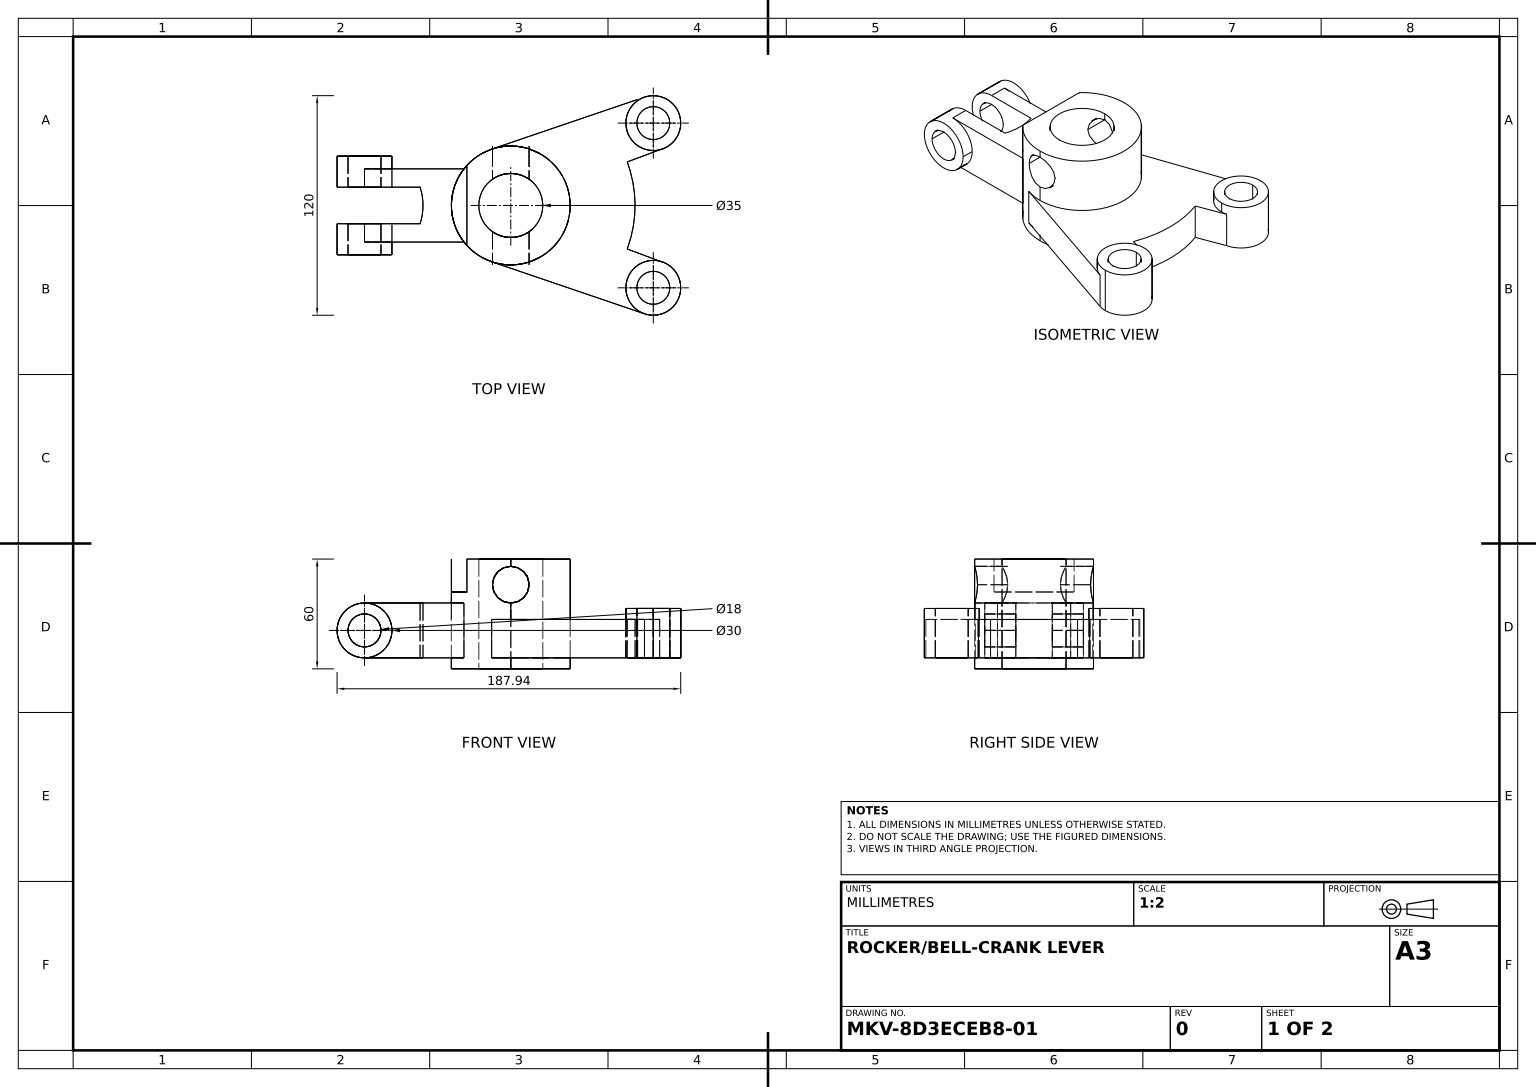
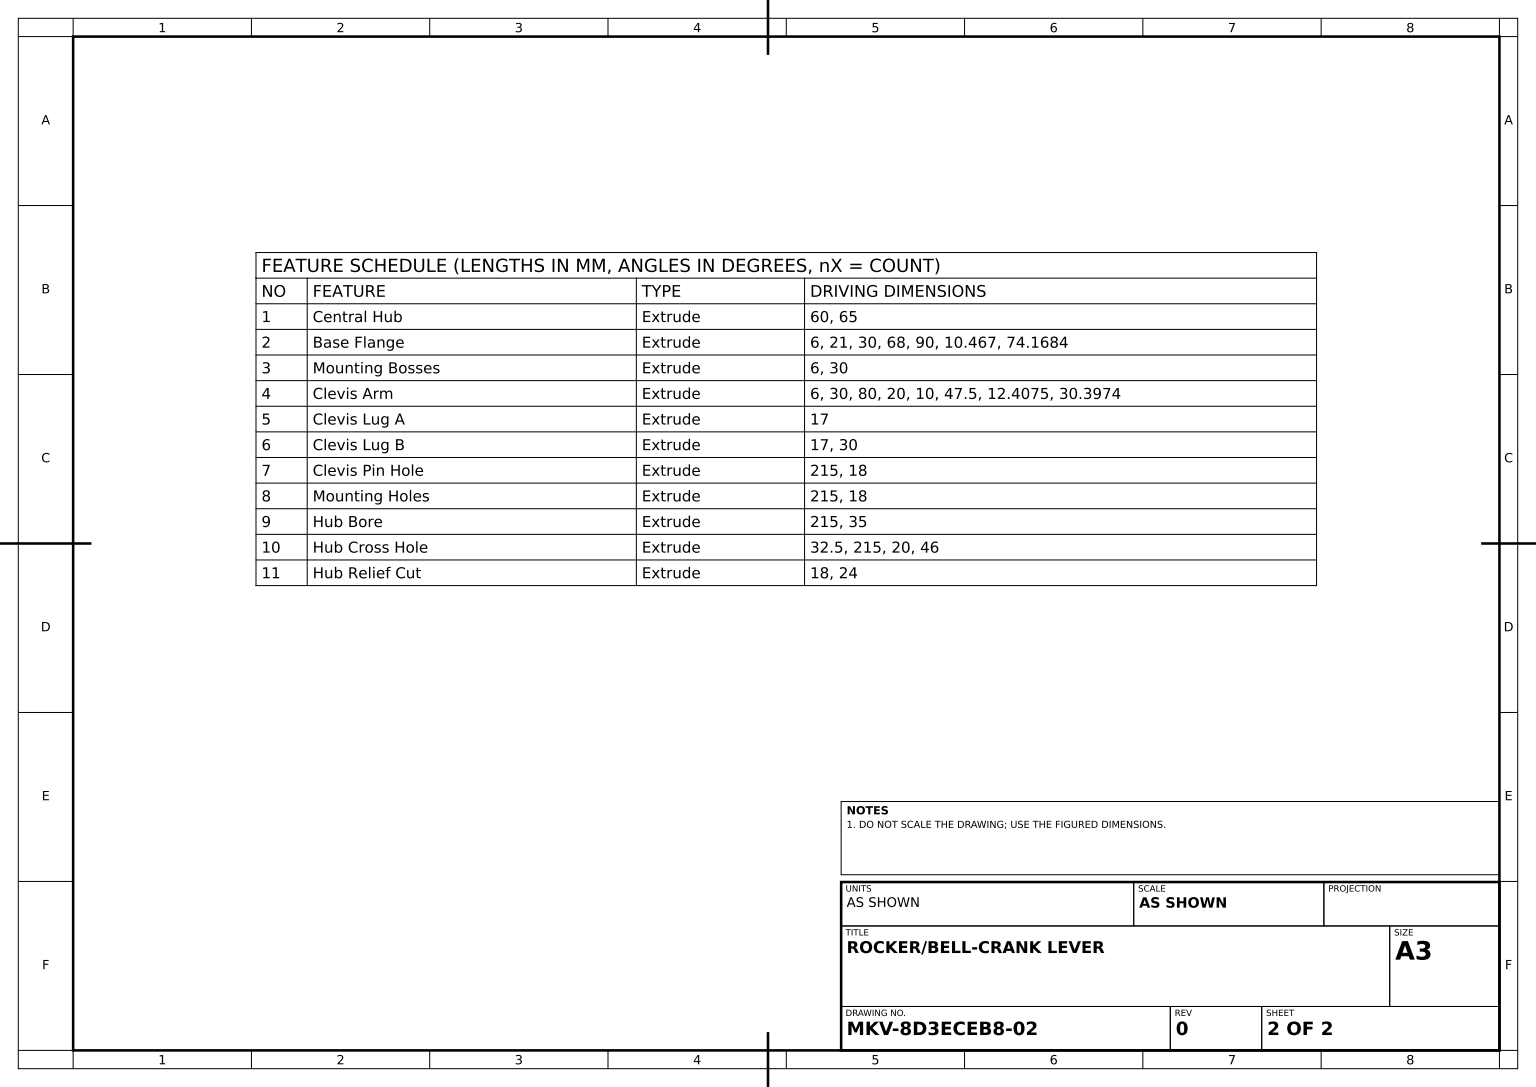
SolidWorks part; units mm, degrees
material "Plain Carbon Steel"
ref_plane "Front Plane" through (0, 0, 0) normal (0, 0, 1) x (1, 0, 0)
ref_plane "Top Plane" through (0, 0, 0) normal (0, 1, 0) x (1, 0, 0)
ref_plane "Right Plane" through (0, 0, 0) normal (1, 0, 0) x (0, 0, -1)
sketch "Hub Profile Sketch" plane through (0, 0, 0) normal (0, 1, 0) x (1, 0, 0)
  circle A0 centre (0, 0) radius 32.5
  dimension "D1" = 65
extrude "Central Hub" add sketch "Hub Profile Sketch" along normal blind 60
ref_plane "Plane1" through (0, 6, 0) normal (0, 1, 0) x (1, 0, 0)
sketch "Base Flange Sketch" plane through (0, 6, 0) normal (0, 1, 0) x (1, 0, 0)
  line L0 (-10.467, 30.7683) -> (73.1113, 59.2008)
  line L1 (63.7014, -23.7936) -> (81.3974, -30.4034)
  line L3 (-10.467, -30.7683) -> (73.1113, -59.2008)
  line L5 (63.7014, 23.7936) -> (81.3974, 30.4034)
  circle A1 centre (77.9423, 45) radius 15
  circle A2 centre (77.9423, -45) radius 15
  circle A3 centre (0, 0) radius 32.5 construction
  arc A4 (-10.467, -30.7683) -> (-10.467, 30.7683) centre (0, 0) ccw
  arc A6 (63.7014, -23.7936) -> (63.7014, 23.7936) centre (0, 0) ccw
  arc A7 (68.9882, -57.7981) -> (69.3858, -57.3202) centre (0, 0) ccw
  arc A8 (69.3858, 57.3202) -> (68.9882, 57.7981) centre (0, 0) ccw
  dimension "D1" = 30
  dimension "D2" = 68
  dimension "D3" = 90
  dimension "D4" = 10.467
  dimension "D5" = 74.1684
extrude "Base Flange" add sketch "Base Flange Sketch" along normal blind 21
sketch "Mounting Bosses Sketch" plane through (0, 27, 0) normal (0, 1, 0) x (1, 0, 0)
  circle A0 centre (77.9423, 45) radius 15
  circle A1 centre (77.9423, -45) radius 15
  dimension "D1" = 30
extrude "Mounting Bosses" add sketch "Mounting Bosses Sketch" along normal blind 6
sketch "Clevis Arm Sketch" plane through (0, 6, 0) normal (0, 1, 0) x (1, 0, 0)
  line L1 (-32.5, 20) -> (-20.0925, 20)
  line L2 (-20.0925, 20) -> (-20.0925, -20)
  line L3 (-20.0925, -20) -> (-32.5, -20)
  line L5 (-80, 20) -> (-80, 10)
  line L6 (-80, 10) -> (-80, 20)
  line L7 (-80, 20) -> (-32.5, 20)
  line L8 (-80, -10) -> (-80, -20)
  line L9 (-80, -20) -> (-32.5, -20)
  line L10 (-80, 10) -> (-49.6026, 10)
  line L11 (-80, -20) -> (-80, -10)
  line L12 (-80, -10) -> (-49.6026, -10)
  arc A1 (-49.6026, -10) -> (-49.6026, 10) centre (-80, 0) ccw
  dimension "D1" = 80
  dimension "D2" = 20
  dimension "D3" = 10
  dimension "D4" = 47.5
  dimension "D5" = 12.4075
  dimension "D6" = 30.3974
extrude "Clevis Arm" add sketch "Clevis Arm Sketch" along normal blind 30 contours A1 L12 L8 L9 L3 L2 L1 L7 L5 L10
sketch "Clevis Lug A Sketch" plane through (0, 0, 10) normal (0, 0, -1) x (-1, 0, 0)
  line L0 (80, 36) -> (80, 6) construction
  circle A0 centre (80, 21) radius 15
extrude "Clevis Lug A" add sketch "Clevis Lug A Sketch" against normal blind 17
sketch "Clevis Lug B Sketch" plane through (0, 0, -10) normal (0, 0, 1) x (1, 0, 0)
  circle A0 centre (-80, 21) radius 15
  dimension "D1" = 30
extrude "Clevis Lug B" add sketch "Clevis Lug B Sketch" against normal blind 17
sketch "Clevis Pin Hole Sketch" plane through (0, 0, 27) normal (0, 0, 1) x (1, 0, 0)
  circle A0 centre (-80, 21) radius 9
  dimension "D1" = 18
extrude "Clevis Pin Hole" cut sketch "Clevis Pin Hole Sketch" against normal blind 215
sketch "Mounting Holes Sketch" plane through (0, 33, 0) normal (0, 1, 0) x (1, 0, 0)
  circle A0 centre (77.9423, 45) radius 9
  circle A1 centre (77.9423, -45) radius 9
  dimension "D1" = 18
extrude "Mounting Holes" cut sketch "Mounting Holes Sketch" against normal blind 215
sketch "Hub Bore Sketch" plane through (0, 60, 0) normal (0, 1, 0) x (1, 0, 0)
  circle A0 centre (0, 0) radius 17.5
  dimension "D1" = 35
extrude "Hub Bore" cut sketch "Hub Bore Sketch" against normal blind 215
ref_plane "Plane3" through (0, 0, 32.5) normal (0, 0, 1) x (1, 0, 0)
sketch "Hub Cross Hole Sketch" plane through (0, 0, 32.5) normal (0, 0, 1) x (1, 0, 0)
  circle A0 centre (0, 46) radius 10
  dimension "D1" = 20
  dimension "D2" = 46
extrude "Hub Cross Hole" cut sketch "Hub Cross Hole Sketch" against normal blind 215
sketch "Hub Relief Cut Sketch" plane through (0, 60, 0) normal (0, 1, 0) x (1, 0, 0)
  line L1 (-24, 0) -> (-24, 21.9146)
  line L2 (-24, 0) -> (-24, -21.9146)
  circle A0 centre (0, 0) radius 32.5 construction
  arc A1 (-24, 21.9146) -> (-24, -21.9146) centre (0, 0) ccw
  circle A2 centre (0, 0) radius 17.5 construction
  dimension "D1" = 24
extrude "Hub Relief Cut" cut sketch "Hub Relief Cut Sketch" against normal blind 18
